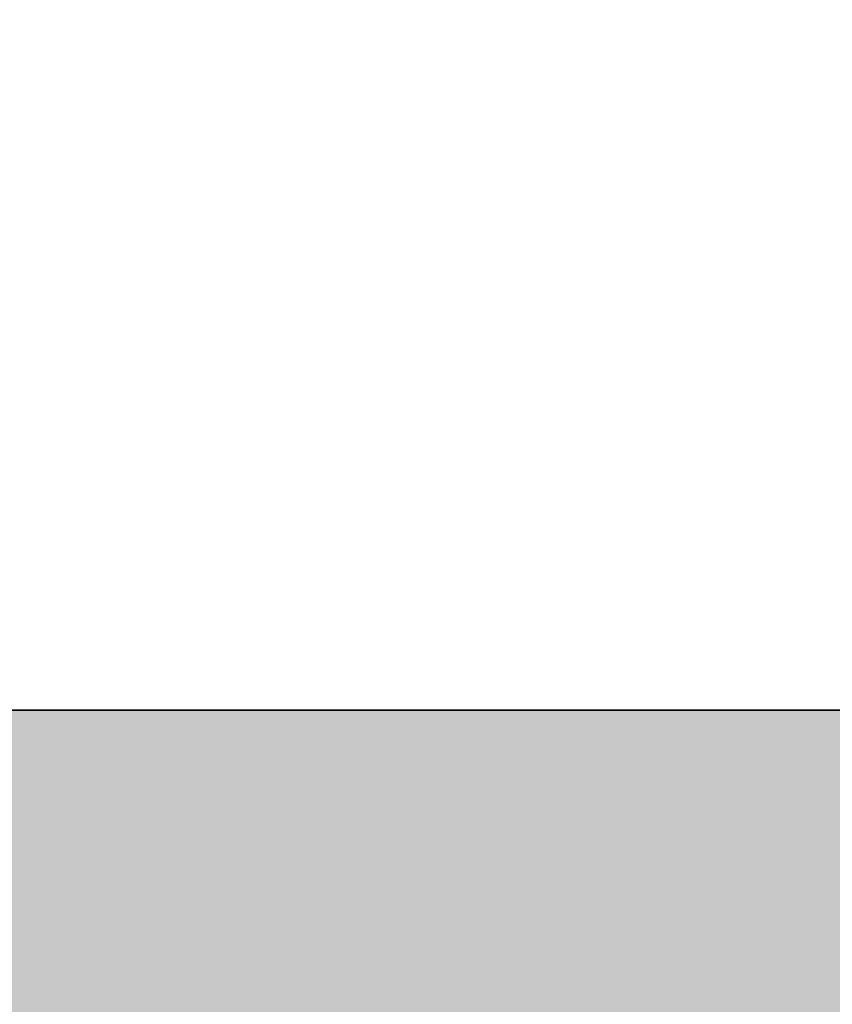
# Model space of a CAD drawing. Units: inches. Extents: x 2083 to 3317, y 1141 to 2115.
# Tile 24 of 256: x 2234.135 to 2235.918, y 1477.116 to 1479.275. Entities that reach past the tile are written whole.
import ezdxf

# ---------------------------------------------------------------- set-up
doc = ezdxf.new("R2010")
doc.units = ezdxf.units.IN
doc.layers.add('A-ANNO-DIMS', color=2, linetype='Continuous', lineweight=18)
doc.layers.add('A-WALL', color=7, linetype='Continuous', lineweight=35)
doc.layers.add('A-WALL-PATT', color=251, linetype='Continuous', lineweight=13, true_color=0x636466)
doc.styles.get("Standard").update_dxf_attribs({"font": 'arial.ttf'})
doc.dimstyles.new('ISO-25', dxfattribs={"dimtxt": 12, "dimasz": 12, "dimexe": 1.25, "dimexo": 0.625, "dimtad": 1, "dimlunit": 3, "dimtxsty": 'Standard', "dimcen": 2.5, "dimadec": 0, "dimazin": 0, "dimtfac": 1, "dimtmove": 0, "dimatfit": 3, "dimfxl": 1, "dimarcsym": 0})

# ---------------------------------------------------------------- blocks, each defined once
blk = doc.blocks.new('*D30')
at = {"layer": 'A-ANNO-DIMS', "color": 0, "lineweight": -2, "transparency": 16777216}
for p, q in [((2240.0179, 1445.2738), (2240.0179, 1448.0455)), ((2254.3293, 1445.2738), (2254.3293, 1448.0455)), ((2228.0179, 1446.7955), (2216.0179, 1446.7955)), ((2240.0179, 1446.7955), (2254.3293, 1446.7955)), ((2266.3293, 1446.7955), (2413.7649, 1446.7955))]:
    blk.add_line(p, q, dxfattribs=at)
at = {"layer": 'A-ANNO-DIMS', "color": 0, "transparency": 16777216}
for points in [[(2228.0179, 1448.7955), (2228.0179, 1444.7955), (2240.0179, 1446.7955)], [(2266.3293, 1448.7955), (2266.3293, 1444.7955), (2254.3293, 1446.7955)]]:
    blk.add_solid(points, dxfattribs=at)
at = {"layer": 'Defpoints', "color": 0, "transparency": 16777216}
for p in [(2254.3293, 1446.7955), (2240.0179, 1444.6488), (2254.3293, 1444.6488)]:
    blk.add_point(p, dxfattribs=at)
at = {"layer": 'A-ANNO-DIMS', "color": 0, "transparency": 16777216, "insert": (2346.0471, 1453.6252), "char_height": 12, "attachment_point": 5}
blk.add_mtext('WC 1\'-2 1/2" TYP.', dxfattribs=at)
blk = doc.blocks.new('*D31')
at = {"layer": 'A-ANNO-DIMS', "color": 0, "lineweight": -2, "transparency": 16777216}
for p, q in [((2237.8711, 1456.6488), (2237.8711, 1541.9152)), ((2239.3929, 1444.6488), (2236.6211, 1444.6488)), ((2237.8711, 1431.5475), (2237.8711, 1444.6488)), ((2239.3929, 1431.5475), (2236.6211, 1431.5475)), ((2237.8711, 1419.5475), (2237.8711, 1407.5475))]:
    blk.add_line(p, q, dxfattribs=at)
at = {"layer": 'A-ANNO-DIMS', "color": 0, "transparency": 16777216}
for points in [[(2235.8711, 1456.6488), (2239.8711, 1456.6488), (2237.8711, 1444.6488)], [(2235.8711, 1419.5475), (2239.8711, 1419.5475), (2237.8711, 1431.5475)]]:
    blk.add_solid(points, dxfattribs=at)
at = {"layer": 'Defpoints', "color": 0, "transparency": 16777216}
for p in [(2237.8711, 1444.6488), (2240.0179, 1444.6488), (2240.0179, 1431.5475)]:
    blk.add_point(p, dxfattribs=at)
at = {"layer": 'A-ANNO-DIMS', "color": 0, "transparency": 16777216, "insert": (2231.2175, 1505.282), "char_height": 12, "attachment_point": 5, "rotation": 90}
blk.add_mtext('1\'-1" TYP.', dxfattribs=at)

msp = doc.modelspace()

# ---------------------------------------------------------------- hatches: boundary and pattern name
at = {"layer": 'A-WALL-PATT'}
h = msp.add_hatch(color=256, dxfattribs=at)
h.dxf.hatch_style = 1
h.paths.add_polyline_path([(3126.9598, 2020.7614), (2748.9598, 2020.7614), (2604.9598, 2020.7614), (2226.9598, 2020.7614), (2226.9598, 1702.7614), (2466.9598, 1702.7614), (2466.9598, 1582.7614), (2418.9598, 1582.7614), (2418.9598, 1477.7614), (2226.9598, 1477.7614), (2226.9598, 1263.2614), (2544.9598, 1263.2614), (2544.9598, 1411.7614), (2604.9598, 1411.7614), (2685.9598, 1411.7614), (2685.9598, 1420.7614), (2604.9598, 1420.7614), (2604.9598, 1573.7614), (2604.9598, 1702.7614), (2604.9598, 2011.7614), (2748.9598, 2011.7614), (2748.9598, 1702.7614), (2862.9598, 1702.7614), (2862.9598, 1621.7614), (2871.9598, 1621.7614), (2871.9598, 1702.7614), (2883.9598, 1702.7614), (2883.9598, 1706.9395, -0.026459), (2883.9598, 1711.7614), (2757.9598, 1711.7614), (2757.9598, 1807.7614), (2787.9598, 1807.7614), (2787.9598, 1812.2614), (2757.9598, 1812.2614), (2757.9598, 2011.7614), (2877.9598, 2011.7614), (2877.9598, 1812.2614), (2847.9598, 1812.2614), (2847.9598, 1807.7614), (2889.8357, 1807.7614), (2889.8357, 1812.2614), (2882.4598, 1812.2614), (2882.4598, 2011.7614), (3117.9598, 2011.7614), (3117.9598, 1812.2614), (2937.8357, 1812.2614), (2937.8357, 1807.7614), (2995.7098, 1807.7614), (2995.7098, 1796.1177), (3000.2098, 1796.1177), (3000.2098, 1807.7614), (3117.9598, 1807.7614), (3117.9598, 1711.7614), (3000.2098, 1711.7614), (3000.2098, 1760.1177), (2998.5727, 1760.1177, -0.020711), (2995.7098, 1760.1177), (2995.7098, 1711.7614), (2931.9598, 1711.7614), (2931.9598, 1702.7614), (3126.9598, 1702.7614)])
h.paths.add_polyline_path([(2471.4598, 2011.7614), (2471.4598, 1810.0114), (2462.7169, 1810.0114), (2462.7169, 1805.5114), (2505.9598, 1805.5114), (2505.9598, 1810.0114), (2475.9598, 1810.0114), (2475.9598, 2011.7614), (2595.9598, 2011.7614), (2595.9598, 1810.0114), (2565.9598, 1810.0114), (2565.9598, 1805.5114), (2595.9598, 1805.5114), (2595.9598, 1711.7614), (2235.9598, 1711.7614), (2235.9598, 1805.5114), (2353.7098, 1805.5114), (2353.7098, 1796.0542), (2358.2098, 1796.0542), (2358.2098, 1805.5114), (2414.7169, 1805.5114), (2414.7169, 1810.0114), (2235.9598, 1810.0114), (2235.9598, 2011.7614)], flags=16)
h.paths.add_polyline_path([(2270.2047, 1994.61), (2270.2047, 1970.61), (2246.2047, 1970.61), (2246.2047, 1994.61)], flags=0)
edge = h.paths.add_edge_path(flags=0)
edge.add_ellipse((2332.0274, 1899.7982), major_axis=(-3.043, 3.043), ratio=0.168252, start_angle=-161.3322, end_angle=-156.3071, ccw=False)
edge.add_ellipse((2333.082, 1898.7435), major_axis=(-1.0546, 1.0546), ratio=0.453532, start_angle=-123.371, end_angle=-94.1591)
edge = h.paths.add_edge_path(flags=0)
edge.add_ellipse((2332.0274, 1968.8763), major_axis=(3.043, 3.043), ratio=0.168252, start_angle=18.6678, end_angle=23.6929)
edge.add_spline(control_points=[(2332.9256, 1970.6911), (2332.2268, 1970.3361), (2330.8937, 1969.6589), (2328.4131, 1970.9321), (2327.2039, 1967.7487), (2324.7096, 1969.9556), (2322.5328, 1967.0124), (2320.0128, 1971.2958), (2317.6803, 1968.1578), (2316.0405, 1967.102), (2315.4269, 1966.8096)], knot_values=[0, 0, 0, 0, 2.267059, 4.324559, 6.685584, 8.878641, 11.121502, 14.300359, 17.755284, 19.732645, 19.732645, 19.732645, 19.732645], degree=3, periodic=0)
edge.add_ellipse((2332.0274, 1968.8763), major_axis=(3.043, 3.043), ratio=0.168252, start_angle=18.6678, end_angle=23.6929, ccw=False)
edge.add_ellipse((2333.082, 1969.9309), major_axis=(1.0546, 1.0546), ratio=0.453532, start_angle=56.629, end_angle=85.8409, ccw=False)
edge = h.paths.add_edge_path(flags=0)
edge.add_spline(control_points=[(2296.4283, 1967.9879), (2293.6278, 1965.3363), (2287.7036, 1959.7271), (2299.7439, 1949.9957), (2294.5326, 1935.6685), (2290.5732, 1920.6035), (2293.3941, 1909.9737), (2296.1854, 1904.9665)], knot_values=[0.099185, 0.099185, 0.099185, 0.099185, 0.345301, 0.619822, 0.982653, 1.386093, 1.810555, 1.810555, 1.810555, 1.810555], degree=3, periodic=0)
edge.add_spline(control_points=[(2296.1854, 1904.9665), (2297.3836, 1902.6193), (2298.001, 1901.9493), (2298.553, 1901.4682)], knot_values=[0.006246, 0.006246, 0.006246, 0.006246, 0.055476, 0.055476, 0.055476, 0.055476], degree=3, periodic=0)
edge.add_spline(control_points=[(2298.553, 1901.4682), (2297.2586, 1900.9232), (2295.2253, 1900.2321), (2293.0602, 1900.6142), (2292.1014, 1900.7884), (2292.0896, 1900.7906)], knot_values=[0.312835, 0.312835, 0.312835, 0.312835, 0.40178, 0.474987, 0.475903, 0.475903, 0.475903, 0.475903], degree=3, periodic=0)
edge.add_arc((2292.7936, 1904.6641), 3.937, 215.4209, 259.6982, ccw=False)
edge.add_spline(control_points=[(2289.5853, 1902.3823), (2289.4767, 1902.5351), (2289.3685, 1902.688), (2289.2609, 1902.8412)], knot_values=[0.102872, 0.102872, 0.102872, 0.102872, 0.116896, 0.116896, 0.116896, 0.116896], degree=3, periodic=0)
edge.add_spline(control_points=[(2289.2609, 1902.8412), (2288.6866, 1902.5502), (2287.64, 1902.0199), (2285.8813, 1901.874), (2283.853, 1901.5044), (2281.72, 1899.7105), (2278.467, 1899.4929), (2276.1571, 1901.8832), (2272.259, 1899.8041), (2267.7776, 1901.8432), (2262.2439, 1900.184), (2257.4149, 1901.7821), (2254.3184, 1900.7261), (2253.1783, 1900.3373)], knot_values=[0, 0, 0, 0, 1.907977, 3.477176, 5.261074, 7.972851, 11.680248, 13.717921, 16.939592, 22.789562, 27.502503, 33.595215, 37.145618, 37.145618, 37.145618, 37.145618], degree=3, periodic=0)
edge.add_line((2253.1783, 1900.3373), (2250.2442, 1902.8412))
edge.add_line((2250.2442, 1902.8412), (2250.2442, 1965.8333))
edge.add_line((2250.2442, 1965.8333), (2253.1783, 1968.3371))
edge.add_spline(control_points=[(2253.1783, 1968.3371), (2254.3184, 1967.9483), (2257.4149, 1966.8924), (2262.2439, 1968.4904), (2267.7776, 1966.8313), (2271.5267, 1968.5372), (2273.8759, 1967.8283), (2274.2067, 1967.7276)], knot_values=[0, 0, 0, 0, 0.09018, 0.244935, 0.364644, 0.513233, 0.537855, 0.537855, 0.537855, 0.537855], degree=3, periodic=0)
edge.add_arc((2274.3529, 1963.7933), 3.937, 72.0511, 92.1279, ccw=False)
edge.add_arc((2281.2969, 1985.23), 18.5963, 252.05113, 288.56572)
edge.add_arc((2292.3167, 1956.0289), 12.6461, 71.02679, 113.77822, ccw=False)
edge = h.paths.add_edge_path(flags=0)
edge.add_spline(control_points=[(2274.8994, 1951.8562), (2275.0662, 1951.6166), (2275.2327, 1951.3766), (2275.398, 1951.1359)], knot_values=[1.409916, 1.409916, 1.409916, 1.409916, 1.43159, 1.43159, 1.43159, 1.43159], degree=3, periodic=0)
edge.add_spline(control_points=[(2275.398, 1951.1359), (2275.7921, 1950.5619), (2276.1792, 1949.9838), (2276.5455, 1949.3971)], knot_values=[1.358238, 1.358238, 1.358238, 1.358238, 1.409916, 1.409916, 1.409916, 1.409916], degree=3, periodic=0)
edge.add_line((2276.5455, 1949.3971), (2277.4373, 1947.8622))
edge.add_spline(control_points=[(2277.4373, 1947.8622), (2276.3038, 1945.6731), (2274.6397, 1942.4269), (2274.6316, 1938.0939), (2272.7991, 1930.8515), (2274.3564, 1943.897), (2275.9477, 1947.9234), (2276.5455, 1949.3971)], knot_values=[0.005632, 0.005632, 0.005632, 0.005632, 0.186014, 0.266002, 0.357087, 0.59639, 0.739732, 0.739732, 0.739732, 0.739732], degree=3, periodic=0)
edge.add_spline(control_points=[(2276.5455, 1949.3971), (2276.1792, 1949.9838), (2275.7921, 1950.5619), (2275.398, 1951.1359)], knot_values=[1.358238, 1.358238, 1.358238, 1.358238, 1.409916, 1.409916, 1.409916, 1.409916], degree=3, periodic=0)
edge.add_spline(control_points=[(2275.398, 1951.1359), (2274.9425, 1950.0805), (2274.2078, 1948.0253), (2273.9346, 1944.8515), (2272.4685, 1937.6275), (2273.4662, 1945.6965), (2274.7006, 1951.0595), (2274.8994, 1951.8562)], knot_values=[0.104364, 0.104364, 0.104364, 0.104364, 0.189636, 0.269624, 0.36071, 0.600013, 0.644622, 0.644622, 0.644622, 0.644622], degree=3, periodic=0)
h.paths.add_polyline_path([(2269.1675, 1963.1276, -0.357527), (2268.1706, 1960.9764, -0.092561), (2268.1706, 1939.4363, -0.357527), (2269.1675, 1937.2851, -0.357527), (2267.0163, 1938.282, -0.164785), (2254.6856, 1938.282, -0.357527), (2252.5344, 1937.2851, -0.357527), (2253.5313, 1939.4363, -0.092561), (2253.5313, 1960.9764, -0.357527), (2252.5344, 1963.1276, -0.357527), (2254.6856, 1962.1307, -0.164785), (2267.0163, 1962.1307, -0.357527)], flags=0)
h.paths.add_polyline_path([(2248.8741, 1967.8018), (2248.8741, 1957.0277), (2249.4578, 1957.0277), (2249.4578, 1911.6468), (2248.8741, 1911.6468), (2248.8741, 1900.8727), (2246.5119, 1900.8727, 0.197327), (2244.1497, 1902.4569), (2244.1497, 1966.2176, 0.197327), (2246.5119, 1967.8018)], flags=0)
h.paths.add_polyline_path([(2269.1675, 1931.3893, -0.357527), (2268.1706, 1929.2381, -0.092561), (2268.1706, 1907.6981, -0.357527), (2269.1675, 1905.5469, -0.357527), (2267.0163, 1906.5438, -0.164785), (2254.6856, 1906.5438, -0.357527), (2252.5344, 1905.5469, -0.357527), (2253.5313, 1907.6981, -0.092561), (2253.5313, 1929.2381, -0.357527), (2252.5344, 1931.3893, -0.357527), (2254.6856, 1930.3925, -0.164785), (2267.0163, 1930.3925, -0.357527)], flags=0)
edge = h.paths.add_edge_path(flags=0)
edge.add_spline(control_points=[(2276.1969, 1906.7237), (2276.1681, 1909.0289), (2276.114, 1913.3719), (2270.5984, 1924.925), (2273.9052, 1919.0128), (2275.9217, 1916.2621), (2275.4746, 1912.4021), (2277.2579, 1910.3806), (2276.696, 1908.225), (2276.6462, 1906.813), (2276.6178, 1906.0084)], knot_values=[0, 0, 0, 0, 8.61026, 16.221274, 18.843057, 23.804898, 27.440828, 29.356102, 31.203478, 33.650687, 33.650687, 33.650687, 33.650687], degree=3, periodic=0)
edge.add_spline(control_points=[(2276.6178, 1906.0084), (2276.6233, 1905.6241), (2276.4977, 1904.6287), (2275.4418, 1903.8547), (2274.9373, 1903.0804), (2274.8591, 1902.8412)], knot_values=[0.156488, 0.156488, 0.156488, 0.156488, 0.184398, 0.231376, 0.250598, 0.250598, 0.250598, 0.250598], degree=3, periodic=0)
edge.add_line((2274.8591, 1902.8412), (2276.506, 1902.8412))
edge.add_spline(control_points=[(2276.506, 1902.8412), (2276.7883, 1903.0849), (2277.6651, 1904.1252), (2278.2495, 1904.3407), (2277.6539, 1908.5274), (2278.1557, 1906.2278), (2278.1005, 1905.2859), (2278.8467, 1904.069), (2277.8568, 1903.4149), (2277.8742, 1902.991), (2277.9036, 1902.8412)], knot_values=[0.059574, 0.059574, 0.059574, 0.059574, 0.080753, 0.103741, 0.16972, 0.176036, 0.207137, 0.240474, 0.262341, 0.27366, 0.27366, 0.27366, 0.27366], degree=3, periodic=0)
edge.add_line((2277.9036, 1902.8412), (2280.0298, 1902.8412))
edge.add_spline(control_points=[(2280.0298, 1902.8412), (2279.8882, 1903.0884), (2279.4993, 1903.9816), (2280.1523, 1905.9393), (2278.1036, 1909.6578), (2279.7624, 1907.1853), (2280.3279, 1904.8749), (2280.4851, 1903.4896), (2281.4633, 1903.2494), (2281.7583, 1902.9365), (2281.834, 1902.8412)], knot_values=[0.013856, 0.013856, 0.013856, 0.013856, 0.034874, 0.088867, 0.107879, 0.126738, 0.158714, 0.193757, 0.217487, 0.226722, 0.226722, 0.226722, 0.226722], degree=3, periodic=0)
edge.add_spline(control_points=[(2281.834, 1902.8412), (2281.7875, 1902.8267), (2281.647, 1902.783), (2281.3955, 1902.8595), (2281.0881, 1902.9852), (2280.7207, 1903.0609), (2280.3335, 1903.0257), (2280.1248, 1902.8989), (2280.0298, 1902.8412)], knot_values=[0, 0, 0, 0, 0.14413, 0.435517, 0.749276, 1.153046, 1.548371, 1.878348, 1.878348, 1.878348, 1.878348], degree=3, periodic=0)
edge.add_line((2280.0298, 1902.8412), (2277.9036, 1902.8412))
edge.add_spline(control_points=[(2277.9036, 1902.8412), (2277.8929, 1902.7959), (2277.8654, 1902.6796), (2277.6075, 1902.6875), (2277.2741, 1902.8007), (2276.8379, 1902.6198), (2276.5838, 1902.7893), (2276.506, 1902.8412)], knot_values=[0, 0, 0, 0, 0.127189, 0.326199, 0.628009, 1.24357, 1.515331, 1.515331, 1.515331, 1.515331], degree=3, periodic=0)
edge.add_line((2276.506, 1902.8412), (2274.8591, 1902.8412))
edge.add_spline(control_points=[(2274.8591, 1902.8412), (2274.8144, 1902.8986), (2274.7251, 1903.0134), (2274.4935, 1903.119), (2274.2443, 1902.9605), (2273.9371, 1903.1849), (2273.614, 1902.9831), (2273.4083, 1902.883), (2273.3223, 1902.8412)], knot_values=[0, 0, 0, 0, 0.21843, 0.436957, 0.687977, 0.990379, 1.398396, 1.69185, 1.69185, 1.69185, 1.69185], degree=3, periodic=0)
edge.add_spline(control_points=[(2273.3223, 1902.8412), (2273.6167, 1903.4457), (2274.274, 1904.5383), (2276.0272, 1904.5737), (2276.207, 1906.5836), (2276.1969, 1906.7237)], knot_values=[0.012227, 0.012227, 0.012227, 0.012227, 0.059472, 0.106218, 0.134458, 0.134458, 0.134458, 0.134458], degree=3, periodic=0)
h.paths.add_polyline_path([(2270.7761, 1897.7898), (2270.7761, 1873.7898), (2246.7761, 1873.7898), (2246.7761, 1897.7898)], flags=0)
h.paths.add_polyline_path([(2353.7098, 1760.0051), (2353.7098, 1760.0542), (2358.2098, 1760.0542, -0.033729)], flags=0)
h.paths.add_polyline_path([(2321.8191, 1737.5292), (2341.9953, 1737.5292, -0.414214), (2343.2033, 1736.3212), (2343.2033, 1721.0206, -0.414214), (2341.9953, 1719.8127), (2321.8191, 1719.8127, -0.414214), (2320.6112, 1721.0206), (2320.6112, 1736.3212, -0.414214)], flags=0)
h.paths.add_polyline_path([(2324.235, 1736.3212), (2339.5794, 1736.3212, -0.414214), (2341.9953, 1733.9053), (2341.9953, 1725.4497, -0.414214), (2339.5794, 1723.0338), (2333.6806, 1723.0338), (2333.8453, 1722.0455, -0.870646), (2335.4254, 1721.8259, -0.767327), (2333.9227, 1721.4232), (2331.291, 1721.4232, -0.767327), (2329.7883, 1721.8259, -0.870646), (2331.3684, 1722.0455), (2331.5331, 1723.0338), (2324.235, 1723.0338, -0.414214), (2321.8191, 1725.4497), (2321.8191, 1733.9053, -0.414214)], flags=0)
h.paths.add_polyline_path([(2570.4838, 1928.6154), (2589.6838, 1928.6154), (2590.1688, 1928.6154), (2590.1688, 1904.9934), (2570.4838, 1904.9934)], flags=0)
h.paths.add_polyline_path([(2574.4473, 1927.2638, -1), (2572.8288, 1927.2638, -1)], flags=0)
h.paths.add_polyline_path([(2573.0899, 1926.9409), (2573.925, 1927.776), (2574.1477, 1927.5533), (2573.3126, 1926.7182)], flags=0)
h.paths.add_polyline_path([(2578.7791, 1919.7296, -1), (2571.5917, 1919.7296, -1)], flags=0)
h.paths.add_polyline_path([(2578.3854, 1919.7296, -1), (2571.9854, 1919.7296, -1)], flags=0)
h.paths.add_polyline_path([(2331.5958, 1729.4762, -1), (2333.618, 1729.4762, -1)], flags=0)
h.paths.add_polyline_path([(2578.0342, 1927.2638, -1), (2576.4157, 1927.2638, -1)], flags=0)
h.paths.add_polyline_path([(2576.6889, 1927.5311), (2576.9116, 1927.7538), (2577.7467, 1926.9186), (2577.524, 1926.6959)], flags=0)
h.paths.add_polyline_path([(2578.1391, 1909.8595, -1), (2572.2317, 1909.8595, -1)], flags=0)
h.paths.add_polyline_path([(2577.7454, 1909.8595, -1), (2572.6254, 1909.8595, -1)], flags=0)
h.paths.add_polyline_path([(2583.7977, 1927.2638, -1), (2582.1792, 1927.2638, -1)], flags=0)
h.paths.add_polyline_path([(2582.7186, 1927.7538), (2583.5538, 1926.9186), (2583.3311, 1926.6959), (2582.4959, 1927.5311)], flags=0)
h.paths.add_polyline_path([(2582.4959, 1927.5311), (2582.7186, 1927.7538), (2583.5538, 1926.9186), (2583.3311, 1926.6959)], flags=0)
h.paths.add_polyline_path([(2587.7391, 1920.5296, -1), (2581.8317, 1920.5296, -1)], flags=0)
h.paths.add_polyline_path([(2587.3454, 1920.5296, -1), (2582.2254, 1920.5296, -1)], flags=0)
h.paths.add_polyline_path([(2587.3846, 1927.2638, -1), (2585.7661, 1927.2638, -1)], flags=0)
h.paths.add_polyline_path([(2586.082, 1926.9802), (2586.9172, 1927.8154), (2587.1399, 1927.5927), (2586.3047, 1926.7575)], flags=0)
h.paths.add_polyline_path([(2588.3791, 1910.6595, -1), (2581.1917, 1910.6595, -1)], flags=0)
h.paths.add_polyline_path([(2587.9854, 1910.6595, -1), (2581.5854, 1910.6595, -1)], flags=0)
h.paths.add_polyline_path([(2417.1677, 1729.4779), (2437.3439, 1729.4779, -0.414214), (2438.5519, 1728.2699), (2438.5519, 1712.9693, -0.414214), (2437.3439, 1711.7614), (2417.1677, 1711.7614, -0.414214), (2415.9598, 1712.9693), (2415.9598, 1728.2699, -0.414214)], flags=0)
h.paths.add_polyline_path([(2419.5836, 1728.2699), (2434.928, 1728.2699, -0.414214), (2437.3439, 1725.8541), (2437.3439, 1717.3984, -0.414214), (2434.928, 1714.9825), (2429.0292, 1714.9825), (2429.1939, 1713.9942, -0.870646), (2430.774, 1713.7746, -0.767327), (2429.2713, 1713.372), (2426.6396, 1713.372, -0.767327), (2425.1369, 1713.7746, -0.870646), (2426.717, 1713.9942), (2426.8817, 1714.9825), (2419.5836, 1714.9825, -0.414214), (2417.1677, 1717.3984), (2417.1677, 1725.8541, -0.414214)], flags=0)
h.paths.add_polyline_path([(2419.5836, 1728.2699), (2434.928, 1728.2699, -0.414214), (2437.3439, 1725.8541), (2437.3439, 1717.3984, -0.414214), (2434.928, 1714.9825), (2429.0292, 1714.9825), (2428.3581, 1719.009), (2427.5528, 1719.009), (2426.8817, 1714.9825), (2419.5836, 1714.9825, -0.414214), (2417.1677, 1717.3984), (2417.1677, 1725.8541, -0.414214)], flags=0)
h.paths.add_polyline_path([(2426.9444, 1721.4249, -1), (2428.9666, 1721.4249, -1)], flags=0)
h.paths.add_polyline_path([(2475.9598, 1702.7614), (2595.9598, 1702.7614), (2595.9598, 1582.7614), (2475.9598, 1582.7614)], flags=16)
h.paths.add_polyline_path([(2427.9598, 1573.7614), (2595.9598, 1573.7614), (2595.9598, 1468.7614), (2595.9598, 1420.7614), (2384.4598, 1420.7614), (2384.4598, 1468.7614), (2427.9598, 1468.7614)], flags=16)
h.paths.add_polyline_path([(2379.9598, 1468.7614), (2379.9598, 1420.7614), (2235.9598, 1420.7614), (2235.9598, 1468.7614)], flags=16)
h.paths.add_polyline_path([(2317.816, 1466.6958), (2337.9922, 1466.6958, -0.414214), (2339.2002, 1465.4878), (2339.2002, 1450.1872, -0.414214), (2337.9922, 1448.9792), (2317.816, 1448.9792, -0.414214), (2316.6081, 1450.1872), (2316.6081, 1465.4878, -0.414214)], flags=0)
h.paths.add_polyline_path([(2320.2319, 1465.4878), (2335.5763, 1465.4878, -0.414214), (2337.9922, 1463.0719), (2337.9922, 1454.6163, -0.414214), (2335.5763, 1452.2004), (2329.6775, 1452.2004), (2329.8422, 1451.212, -0.870646), (2331.4223, 1450.9925, -0.767327), (2329.9196, 1450.5898), (2327.2879, 1450.5898, -0.767327), (2325.7852, 1450.9925, -0.870646), (2327.3653, 1451.212), (2327.53, 1452.2004), (2320.2319, 1452.2004, -0.414214), (2317.816, 1454.6163), (2317.816, 1463.0719, -0.414214)], flags=0)
h.paths.add_polyline_path([(2320.2319, 1465.4878), (2335.5763, 1465.4878, -0.414214), (2337.9922, 1463.0719), (2337.9922, 1454.6163, -0.414214), (2335.5763, 1452.2004), (2329.6775, 1452.2004), (2329.0064, 1456.2269), (2328.2011, 1456.2269), (2327.53, 1452.2004), (2320.2319, 1452.2004, -0.414214), (2317.816, 1454.6163), (2317.816, 1463.0719, -0.414214)], flags=0)
h.paths.add_polyline_path([(2327.5926, 1458.6428, -1), (2329.6148, 1458.6428, -1)], flags=0)
h.paths.add_polyline_path([(2244.4117, 1433.3405), (2241.9209, 1433.3405, -0.414214), (2240.0179, 1435.2435), (2240.0179, 1440.9528, -0.414211), (2241.9209, 1442.8559), (2244.4117, 1442.8559, -1.976472)], flags=0)
h.paths.add_polyline_path([(2245.3569, 1434.3975, -0.414214), (2245.3569, 1441.7988, -2.144098)], flags=0)
h.paths.add_polyline_path([(2535.9598, 1416.2614), (2535.9598, 1272.2614), (2235.9598, 1272.2614), (2235.9598, 1416.2614)], flags=16)
h.paths.add_polyline_path([(2260.1196, 1384.2928), (2260.1196, 1362.0386), (2237.8654, 1362.0386), (2237.8654, 1384.2928)], flags=0)
edge = h.paths.add_edge_path(flags=0)
edge.add_line((2318.2518, 1362.0933), (2318.1458, 1362.001))
edge.add_ellipse((2317.4451, 1360.431), major_axis=(2.8216, 2.8216), ratio=0.168252, start_angle=18.6678, end_angle=20.9481, ccw=False)
edge.add_ellipse((2318.423, 1361.409), major_axis=(0.9779, 0.9779), ratio=0.453532, start_angle=56.629, end_angle=70.2262, ccw=False)
edge = h.paths.add_edge_path(flags=0)
edge.add_line((2319.1074, 1295.5711), (2319.015, 1295.6771))
edge.add_ellipse((2317.4451, 1296.3778), major_axis=(-2.8216, 2.8216), ratio=0.168252, start_angle=-161.3322, end_angle=-159.0519, ccw=False)
edge.add_ellipse((2318.423, 1295.3999), major_axis=(-0.9779, 0.9779), ratio=0.453532, start_angle=-123.371, end_angle=-109.7738)
edge = h.paths.add_edge_path(flags=0)
edge.add_spline(control_points=[(2284.2103, 1301.1702), (2284.5807, 1300.4447), (2284.8912, 1299.892), (2285.1596, 1299.461)], knot_values=[0.039066, 0.039066, 0.039066, 0.039066, 0.055476, 0.055476, 0.055476, 0.055476], degree=3, periodic=0)
edge.add_line((2285.1596, 1299.461), (2284.2103, 1301.1702))
edge = h.paths.add_edge_path(flags=0)
edge.add_line((2280.4125, 1297.298), (2283.37, 1297.0361))
edge.add_line((2283.37, 1297.0361), (2286.4057, 1297.9263))
edge.add_spline(control_points=[(2286.4057, 1297.9263), (2285.3055, 1297.4631), (2284.3448, 1297.1292), (2283.37, 1297.0361)], knot_values=[0.394369, 0.394369, 0.394369, 0.394369, 0.475903, 0.475903, 0.475903, 0.475903], degree=3, periodic=0)
edge.add_spline(control_points=[(2283.37, 1297.0361), (2283.2814, 1297.0277), (2282.3163, 1296.9573), (2281.3125, 1297.1345), (2280.4234, 1297.296), (2280.4125, 1297.298)], knot_values=[0.312835, 0.312835, 0.312835, 0.312835, 0.320246, 0.393453, 0.394369, 0.394369, 0.394369, 0.394369], degree=3, periodic=0)
edge = h.paths.add_edge_path(flags=0)
edge.add_line((2284.4356, 1359.6073), (2280.4463, 1355.328))
edge.add_line((2280.4463, 1355.328), (2279.58, 1351.0178))
edge.add_line((2279.58, 1351.0178), (2282.413, 1346.5804))
edge.add_spline(control_points=[(2282.413, 1346.5804), (2283.1533, 1345.5892), (2284.2529, 1344.0289), (2284.801, 1342.3872), (2284.9352, 1341.8055)], knot_values=[1.240098, 1.240098, 1.240098, 1.240098, 1.332892, 1.382712, 1.382712, 1.382712, 1.382712], degree=3, periodic=0)
edge.add_spline(control_points=[(2284.9352, 1341.8055), (2285.3191, 1340.1406), (2285.233, 1338.4092), (2284.9099, 1336.6541)], knot_values=[1.097484, 1.097484, 1.097484, 1.097484, 1.240098, 1.240098, 1.240098, 1.240098], degree=3, periodic=0)
edge.add_spline(control_points=[(2284.9099, 1336.6541), (2284.5868, 1334.899), (2284.0267, 1333.1203), (2283.4626, 1331.3606)], knot_values=[0.95487, 0.95487, 0.95487, 0.95487, 1.097484, 1.097484, 1.097484, 1.097484], degree=3, periodic=0)
edge.add_line((2283.4626, 1331.3606), (2281.8904, 1326.1534))
edge.add_line((2281.8904, 1326.1534), (2280.7563, 1321.0561))
edge.add_line((2280.7563, 1321.0561), (2280.2992, 1316.002))
edge.add_line((2280.2992, 1316.002), (2280.7159, 1310.9501))
edge.add_line((2280.7159, 1310.9501), (2282.0281, 1305.9721))
edge.add_line((2282.0281, 1305.9721), (2284.2103, 1301.1702))
edge.add_spline(control_points=[(2284.2103, 1301.1702), (2283.3407, 1302.7302), (2282.6119, 1304.3365), (2282.0281, 1305.9721)], knot_values=[0.099185, 0.099185, 0.099185, 0.099185, 0.241799, 0.241799, 0.241799, 0.241799], degree=3, periodic=0)
edge.add_spline(control_points=[(2282.0281, 1305.9721), (2281.4443, 1307.6078), (2281.0055, 1309.2728), (2280.7159, 1310.9501)], knot_values=[0.241799, 0.241799, 0.241799, 0.241799, 0.384413, 0.384413, 0.384413, 0.384413], degree=3, periodic=0)
edge.add_spline(control_points=[(2280.7159, 1310.9501), (2280.4332, 1312.5876), (2280.2894, 1314.277), (2280.2989, 1315.962), (2280.2992, 1316.002)], knot_values=[0.384413, 0.384413, 0.384413, 0.384413, 0.523647, 0.527028, 0.527028, 0.527028, 0.527028], degree=3, periodic=0)
edge.add_spline(control_points=[(2280.2992, 1316.002), (2280.3123, 1317.687), (2280.4779, 1319.3679), (2280.7563, 1321.0561)], knot_values=[0.527028, 0.527028, 0.527028, 0.527028, 0.669642, 0.669642, 0.669642, 0.669642], degree=3, periodic=0)
edge.add_spline(control_points=[(2280.7563, 1321.0561), (2281.0346, 1322.7443), (2281.4259, 1324.4396), (2281.8904, 1326.1534)], knot_values=[0.669642, 0.669642, 0.669642, 0.669642, 0.812256, 0.812256, 0.812256, 0.812256], degree=3, periodic=0)
edge.add_spline(control_points=[(2281.8904, 1326.1534), (2282.2644, 1327.5333), (2282.7879, 1329.2618), (2283.3528, 1331.0178), (2283.4626, 1331.3606)], knot_values=[0.812256, 0.812256, 0.812256, 0.812256, 0.927087, 0.95487, 0.95487, 0.95487, 0.95487], degree=3, periodic=0)
edge.add_line((2283.4626, 1331.3606), (2284.9099, 1336.6541))
edge.add_line((2284.9099, 1336.6541), (2284.9352, 1341.8055))
edge.add_line((2284.9352, 1341.8055), (2282.413, 1346.5804))
edge.add_spline(control_points=[(2282.413, 1346.5804), (2281.2751, 1348.1038), (2280.0784, 1349.5703), (2279.58, 1351.0178)], knot_values=[1.382712, 1.382712, 1.382712, 1.382712, 1.525326, 1.525326, 1.525326, 1.525326], degree=3, periodic=0)
edge.add_spline(control_points=[(2279.58, 1351.0178), (2279.4433, 1351.4147), (2279.1363, 1352.8569), (2279.7352, 1354.2904), (2280.4463, 1355.328)], knot_values=[1.525326, 1.525326, 1.525326, 1.525326, 1.564439, 1.667941, 1.667941, 1.667941, 1.667941], degree=3, periodic=0)
edge.add_spline(control_points=[(2280.4463, 1355.328), (2281.4261, 1356.7578), (2282.9308, 1358.1826), (2284.4356, 1359.6073)], knot_values=[1.667941, 1.667941, 1.667941, 1.667941, 1.810555, 1.810555, 1.810555, 1.810555], degree=3, periodic=0)
edge.add_arc((2280.6231, 1348.5182), 11.7262, 71.02679, 113.77822)
edge.add_arc((2270.4049, 1375.5952), 17.2436, 252.05113, 288.56572, ccw=False)
edge.add_arc((2263.966, 1355.7178), 3.6506, 72.0511, 92.1279)
edge.add_arc((2263.966, 1355.7178), 3.6506, 92.1279, 177.9851)
edge.add_spline(control_points=[(2260.3176, 1355.8462), (2260.2604, 1354.2207), (2260.5513, 1350.1865), (2262.9993, 1346.7663), (2264.4727, 1344.649)], knot_values=[1.43159, 1.43159, 1.43159, 1.43159, 1.564144, 1.770695, 1.770695, 1.770695, 1.770695], degree=3, periodic=0)
edge.add_line((2264.4727, 1344.649), (2264.9356, 1343.9825))
edge.add_spline(control_points=[(2263.801, 1340.2481), (2263.8432, 1340.5141), (2264.0672, 1341.7565), (2264.5127, 1343.0025), (2264.935, 1343.9811)], knot_values=[0.53657, 0.53657, 0.53657, 0.53657, 0.559349, 0.644622, 0.644622, 0.644622, 0.644622], degree=3, periodic=0)
edge.add_spline(control_points=[(2264.935, 1343.9811), (2265.1178, 1343.715), (2265.2989, 1343.4479), (2265.4768, 1343.1794)], knot_values=[1.384077, 1.384077, 1.384077, 1.384077, 1.409916, 1.409916, 1.409916, 1.409916], degree=3, periodic=0)
edge.add_spline(control_points=[(2265.4768, 1343.1794), (2265.6546, 1342.9108), (2265.8293, 1342.6408), (2265.9991, 1342.3688)], knot_values=[1.358238, 1.358238, 1.358238, 1.358238, 1.384077, 1.384077, 1.384077, 1.384077], degree=3, periodic=0)
edge.add_line((2265.9991, 1342.3688), (2266.826, 1340.9455))
edge.add_spline(control_points=[(2266.826, 1340.9455), (2268.8944, 1337.0897), (2271.3982, 1325.843), (2270.5162, 1310.5686), (2275.9194, 1301.8606), (2277.7895, 1299.1994)], knot_values=[0.116896, 0.116896, 0.116896, 0.116896, 0.472987, 1.050969, 1.313793, 1.313793, 1.313793, 1.313793], degree=3, periodic=0)
edge.add_spline(control_points=[(2277.7895, 1299.1994), (2277.8394, 1299.1285), (2277.8894, 1299.0575), (2277.9396, 1298.9866)], knot_values=[0.109884, 0.109884, 0.109884, 0.109884, 0.116896, 0.116896, 0.116896, 0.116896], degree=3, periodic=0)
edge.add_line((2277.9396, 1298.9866), (2277.7888, 1299.1991))
edge.add_spline(control_points=[(2277.7888, 1299.1991), (2277.2566, 1298.9294), (2276.2864, 1298.4379), (2275.0394, 1298.3344), (2274.3833, 1298.2389), (2274.2153, 1298.2093)], knot_values=[33.12187, 33.12187, 33.12187, 33.12187, 35.029056, 36.598255, 37.144827, 37.144827, 37.144827, 37.144827], degree=3, periodic=0)
edge.add_line((2274.2153, 1298.2093), (2273.0731, 1297.893))
edge.add_spline(control_points=[(2273.0731, 1297.893), (2272.3229, 1297.5798), (2271.0392, 1296.5105), (2269.2484, 1296.2261), (2268.4231, 1296.3747)], knot_values=[26.532584, 26.532584, 26.532584, 26.532584, 29.198919, 31.839101, 31.839101, 31.839101, 31.839101], degree=3, periodic=0)
edge.add_line((2268.4231, 1296.3747), (2263.8785, 1297.4575))
edge.add_spline(control_points=[(2263.8785, 1297.4575), (2263.5561, 1297.3594), (2261.8603, 1296.8387), (2260.2388, 1297.2824), (2258.9335, 1297.5165)], knot_values=[15.919551, 15.919551, 15.919551, 15.919551, 16.939592, 21.226067, 21.226067, 21.226067, 21.226067], degree=3, periodic=0)
edge.add_line((2258.9335, 1297.5165), (2254.0552, 1297.329))
edge.add_spline(control_points=[(2254.0552, 1297.329), (2253.7555, 1297.2958), (2252.1137, 1297.1652), (2250.4619, 1297.5442), (2249.1297, 1297.6679)], knot_values=[5.306517, 5.306517, 5.306517, 5.306517, 6.276435, 10.613034, 10.613034, 10.613034, 10.613034], degree=3, periodic=0)
edge.add_line((2249.1297, 1297.6679), (2244.3316, 1296.8778))
edge.add_line((2244.3316, 1296.8778), (2241.611, 1299.1994))
edge.add_line((2241.611, 1299.1994), (2241.611, 1357.6094))
edge.add_line((2241.611, 1357.6094), (2244.3316, 1359.9311))
edge.add_line((2244.3316, 1359.9311), (2252.7288, 1359.5427))
edge.add_spline(control_points=[(2252.7288, 1359.5427), (2252.8709, 1359.5464), (2253.3057, 1359.5482), (2253.7398, 1359.5143), (2254.0317, 1359.4824)], knot_values=[0.233291, 0.233291, 0.233291, 0.233291, 0.244935, 0.268927, 0.268927, 0.268927, 0.268927], degree=3, periodic=0)
edge.add_line((2254.0317, 1359.4824), (2259.5872, 1359.4164))
edge.add_spline(control_points=[(2259.5872, 1359.4164), (2260.6771, 1359.6285), (2262.0732, 1359.897), (2263.5237, 1359.4593), (2263.8304, 1359.366)], knot_values=[0.422516, 0.422516, 0.422516, 0.422516, 0.513233, 0.537855, 0.537855, 0.537855, 0.537855], degree=3, periodic=0)
edge.add_arc((2263.966, 1355.7178), 3.6506, 72.0511, 92.1279, ccw=False)
edge.add_arc((2270.4049, 1375.5952), 17.2436, 252.05113, 288.56572)
edge.add_arc((2280.6231, 1348.5182), 11.7262, 71.02679, 113.77822, ccw=False)
h.paths.add_polyline_path([(2240.3405, 1359.4347), (2240.3405, 1349.4444), (2240.8818, 1349.4444), (2240.8818, 1307.3645), (2240.3405, 1307.3645), (2240.3405, 1297.3741), (2238.1502, 1297.3741, 0.197327), (2235.9598, 1298.8431), (2235.9598, 1357.9657, 0.197327), (2238.1502, 1359.4347)], flags=0)
h.paths.add_polyline_path([(2259.1578, 1355.1005, -0.357527), (2258.2334, 1353.1058, -0.092561), (2258.2334, 1333.1326, -0.357527), (2259.1578, 1331.1379, -0.357527), (2257.1631, 1332.0622, -0.164785), (2245.7293, 1332.0622, -0.357527), (2243.7346, 1331.1379, -0.357527), (2244.6589, 1333.1326, -0.092561), (2244.6589, 1353.1058, -0.357527), (2243.7346, 1355.1005, -0.357527), (2245.7293, 1354.1761, -0.164785), (2257.1631, 1354.1761, -0.357527)], flags=0)
edge = h.paths.add_edge_path(flags=0)
edge.add_line((2265.9991, 1342.3688), (2266.826, 1340.9455))
edge.add_line((2266.826, 1340.9455), (2265.3076, 1337.8141))
edge.add_line((2265.3076, 1337.8141), (2264.3582, 1334.6529))
edge.add_line((2264.3582, 1334.6529), (2264.262, 1333.7997))
edge.add_spline(control_points=[(2264.262, 1333.7997), (2264.2084, 1333.1871), (2264.1621, 1332.3655), (2264.0071, 1331.4139), (2263.969, 1331.2018)], knot_values=[0.464444, 0.464444, 0.464444, 0.464444, 0.516691, 0.531608, 0.531608, 0.531608, 0.531608], degree=3, periodic=0)
edge.add_spline(control_points=[(2263.969, 1331.2018), (2263.7745, 1330.1189), (2263.4244, 1328.7908), (2263.2574, 1328.5307), (2263.234, 1328.5146)], knot_values=[0.372682, 0.372682, 0.372682, 0.372682, 0.44885, 0.464444, 0.464444, 0.464444, 0.464444], degree=3, periodic=0)
edge.add_spline(control_points=[(2263.234, 1328.5146), (2263.0964, 1328.4202), (2263.1312, 1329.3015), (2263.275, 1330.6157)], knot_values=[0.280919, 0.280919, 0.280919, 0.280919, 0.372682, 0.372682, 0.372682, 0.372682], degree=3, periodic=0)
edge.add_spline(control_points=[(2263.275, 1330.6157), (2263.4187, 1331.93), (2263.6715, 1333.6773), (2263.9699, 1335.315)], knot_values=[0.189157, 0.189157, 0.189157, 0.189157, 0.280919, 0.280919, 0.280919, 0.280919], degree=3, periodic=0)
edge.add_spline(control_points=[(2263.9699, 1335.315), (2264.1005, 1336.0322), (2264.4188, 1337.6219), (2264.7548, 1338.8644), (2264.9474, 1339.4911)], knot_values=[0.097394, 0.097394, 0.097394, 0.097394, 0.137578, 0.189157, 0.189157, 0.189157, 0.189157], degree=3, periodic=0)
edge.add_spline(control_points=[(2264.9474, 1339.4911), (2265.29, 1340.6061), (2265.6442, 1341.494), (2265.9991, 1342.3688)], knot_values=[0.005632, 0.005632, 0.005632, 0.005632, 0.097394, 0.097394, 0.097394, 0.097394], degree=3, periodic=0)
h.paths.add_polyline_path([(2259.1578, 1325.671, -0.357527), (2258.2334, 1323.6763, -0.092561), (2258.2334, 1303.7031, -0.357527), (2259.1578, 1301.7084, -0.357527), (2257.1631, 1302.6327, -0.164785), (2245.7293, 1302.6327, -0.357527), (2243.7346, 1301.7084, -0.357527), (2244.6589, 1303.7031, -0.092561), (2244.6589, 1323.6763, -0.357527), (2243.7346, 1325.671, -0.357527), (2245.7293, 1324.7466, -0.164785), (2257.1631, 1324.7466, -0.357527)], flags=0)
edge = h.paths.add_edge_path(flags=0)
edge.add_spline(control_points=[(2261.7089, 1317.3114), (2261.6795, 1317.4176), (2261.7619, 1317.3885), (2262.4907, 1316.0899), (2262.9622, 1315.3009)], knot_values=[14.955861, 14.955861, 14.955861, 14.955861, 16.221274, 18.694826, 18.694826, 18.694826, 18.694826], degree=3, periodic=0)
edge.add_spline(control_points=[(2262.9622, 1315.3009), (2262.9904, 1315.2536), (2263.7021, 1314.0674), (2264.349, 1313.1272), (2264.7301, 1312.1642)], knot_values=[18.694826, 18.694826, 18.694826, 18.694826, 18.843057, 22.433791, 22.433791, 22.433791, 22.433791], degree=3, periodic=0)
edge.add_spline(control_points=[(2264.7301, 1312.1642), (2264.8756, 1311.7964), (2265.1769, 1310.7698), (2265.1431, 1309.5593), (2265.2477, 1308.8242)], knot_values=[22.433791, 22.433791, 22.433791, 22.433791, 23.804898, 26.172756, 26.172756, 26.172756, 26.172756], degree=3, periodic=0)
edge.add_line((2265.2477, 1308.8242), (2265.8508, 1307.1719))
edge.add_spline(control_points=[(2265.8508, 1307.1719), (2266.065, 1306.8217), (2266.3844, 1306.3322), (2266.4244, 1305.7805), (2266.4204, 1305.6112)], knot_values=[28.062562, 28.062562, 28.062562, 28.062562, 29.356102, 29.911721, 29.911721, 29.911721, 29.911721], degree=3, periodic=0)
edge.add_spline(control_points=[(2266.4204, 1305.6112), (2266.4161, 1305.4326), (2266.394, 1305.25), (2266.3648, 1305.0659)], knot_values=[29.911721, 29.911721, 29.911721, 29.911721, 30.497837, 30.497837, 30.497837, 30.497837], degree=3, periodic=0)
edge.add_line((2266.3648, 1305.0659), (2266.0662, 1302.1363))
edge.add_spline(control_points=[(2266.0662, 1302.1363), (2266.0712, 1301.78), (2265.9981, 1301.2), (2265.6633, 1300.759), (2265.5089, 1300.5859)], knot_values=[0.156488, 0.156488, 0.156488, 0.156488, 0.184398, 0.203543, 0.203543, 0.203543, 0.203543], degree=3, periodic=0)
edge.add_line((2265.5089, 1300.5859), (2264.4353, 1299.1994))
edge.add_line((2264.4353, 1299.1994), (2265.9624, 1299.1994))
edge.add_line((2265.9624, 1299.1994), (2267.336, 1301.1753))
edge.add_line((2267.336, 1301.1753), (2267.3117, 1301.9862))
edge.add_spline(control_points=[(2267.3117, 1301.9862), (2267.2611, 1302.8624), (2267.1602, 1303.7371), (2267.2715, 1303.3259)], knot_values=[0.126229, 0.126229, 0.126229, 0.126229, 0.166617, 0.166617, 0.166617, 0.166617], degree=3, periodic=0)
edge.add_spline(control_points=[(2267.2715, 1303.3259), (2267.28, 1303.2943), (2267.3098, 1303.1754), (2267.3735, 1302.8836), (2267.4061, 1302.6828), (2267.4179, 1302.601)], knot_values=[0.166617, 0.166617, 0.166617, 0.166617, 0.16972, 0.176036, 0.180765, 0.180765, 0.180765, 0.180765], degree=3, periodic=0)
edge.add_spline(control_points=[(2267.7439, 1300.9875), (2267.6876, 1301.1509), (2267.4805, 1301.6567), (2267.4838, 1302.1448), (2267.4179, 1302.601)], knot_values=[0.180765, 0.180765, 0.180765, 0.180765, 0.193767, 0.220139, 0.220139, 0.220139, 0.220139], degree=3, periodic=0)
edge.add_line((2267.4179, 1302.601), (2267.7439, 1300.9875))
edge.add_spline(control_points=[(2267.7439, 1300.9875), (2267.832, 1300.7319), (2267.932, 1300.3099), (2267.5548, 1299.9745), (2267.4294, 1299.8292)], knot_values=[0.220139, 0.220139, 0.220139, 0.220139, 0.240474, 0.25489, 0.25489, 0.25489, 0.25489], degree=3, periodic=0)
edge.add_line((2267.4294, 1299.8292), (2267.2584, 1299.1994))
edge.add_line((2267.2584, 1299.1994), (2269.23, 1299.1994))
edge.add_spline(control_points=[(2269.23, 1299.1994), (2269.0987, 1299.4287), (2268.8428, 1300.0163), (2269.0116, 1300.9159), (2268.9468, 1301.6607)], knot_values=[0.013856, 0.013856, 0.013856, 0.013856, 0.034874, 0.067073, 0.067073, 0.067073, 0.067073], degree=3, periodic=0)
edge.add_line((2268.9468, 1301.6607), (2268.4316, 1303.6031))
edge.add_spline(control_points=[(2268.4316, 1303.6031), (2268.1756, 1304.1924), (2267.5962, 1305.2513), (2268.0407, 1304.6232), (2268.2514, 1304.2824)], knot_values=[0.090155, 0.090155, 0.090155, 0.090155, 0.107879, 0.120289, 0.120289, 0.120289, 0.120289], degree=3, periodic=0)
edge.add_spline(control_points=[(2268.2514, 1304.2824), (2268.3609, 1304.1053), (2269.0578, 1302.918), (2269.3827, 1301.5904), (2269.5214, 1300.7759), (2269.5752, 1300.5558)], knot_values=[0.120289, 0.120289, 0.120289, 0.120289, 0.126738, 0.158714, 0.173506, 0.173506, 0.173506, 0.173506], degree=3, periodic=0)
edge.add_line((2269.5752, 1300.5558), (2270.6858, 1299.4213))
edge.add_spline(control_points=[(2270.6858, 1299.4213), (2270.7672, 1299.3573), (2270.8379, 1299.2814), (2270.9029, 1299.1994)], knot_values=[0.21816, 0.21816, 0.21816, 0.21816, 0.226722, 0.226722, 0.226722, 0.226722], degree=3, periodic=0)
edge.add_line((2270.9372, 1299.1929), (2270.9029, 1299.1994))
edge.add_spline(control_points=[(2270.9029, 1299.1994), (2270.8598, 1299.186), (2270.7295, 1299.1455), (2270.4963, 1299.2164), (2270.2717, 1299.3083), (2270.121, 1299.348), (2270.0633, 1299.3596)], knot_values=[0.939174, 0.939174, 0.939174, 0.939174, 1.083304, 1.374691, 1.68845, 1.878348, 1.878348, 1.878348, 1.878348], degree=3, periodic=0)
edge.add_line((2270.0633, 1299.3596), (2269.23, 1299.1994))
edge.add_line((2269.23, 1299.1994), (2267.2584, 1299.1994))
edge.add_spline(control_points=[(2267.2584, 1299.1994), (2267.2484, 1299.1574), (2267.223, 1299.0497), (2266.9838, 1299.0569), (2266.8092, 1299.1162), (2266.6769, 1299.1091), (2266.6365, 1299.1048)], knot_values=[0.757665, 0.757665, 0.757665, 0.757665, 0.884854, 1.083864, 1.385675, 1.515331, 1.515331, 1.515331, 1.515331], degree=3, periodic=0)
edge.add_spline(control_points=[(2266.6365, 1299.1048), (2266.4852, 1299.0888), (2266.2358, 1299.0171), (2266.0346, 1299.1513), (2265.9624, 1299.1994)], knot_values=[0, 0, 0, 0, 0.485905, 0.757665, 0.757665, 0.757665, 0.757665], degree=3, periodic=0)
edge.add_line((2265.9624, 1299.1994), (2264.4353, 1299.1994))
edge.add_line((2264.4353, 1299.1994), (2263.8584, 1299.3671))
edge.add_spline(control_points=[(2263.8584, 1299.3671), (2263.8189, 1299.3709), (2263.7795, 1299.3857), (2263.7401, 1299.4015)], knot_values=[0.845925, 0.845925, 0.845925, 0.845925, 0.978627, 0.978627, 0.978627, 0.978627], degree=3, periodic=0)
edge.add_line((2263.7218, 1299.3964), (2263.0103, 1299.1994))
edge.add_spline(control_points=[(2263.0103, 1299.1994), (2263.2458, 1299.6829), (2263.506, 1300.1281), (2263.8735, 1300.408)], knot_values=[0.012227, 0.012227, 0.012227, 0.012227, 0.052971, 0.052971, 0.052971, 0.052971], degree=3, periodic=0)
edge.add_spline(control_points=[(2263.8735, 1300.408), (2263.9321, 1300.4527), (2264.0842, 1300.553), (2264.2552, 1300.6242), (2264.3597, 1300.6647)], knot_values=[0.052971, 0.052971, 0.052971, 0.052971, 0.059472, 0.069086, 0.069086, 0.069086, 0.069086], degree=3, periodic=0)
edge.add_line((2264.3597, 1300.6647), (2265.1419, 1301.0778))
edge.add_line((2265.1419, 1301.0778), (2265.6758, 1302.7996))
edge.add_line((2265.6758, 1302.7996), (2265.5407, 1305.7041))
edge.add_line((2265.5407, 1305.7041), (2264.8031, 1309.3277))
edge.add_line((2264.8031, 1309.3277), (2263.0405, 1314.0918))
edge.add_spline(control_points=[(2263.0405, 1314.0918), (2262.3836, 1315.6714), (2261.796, 1316.9977), (2261.7089, 1317.3114)], knot_values=[11.216896, 11.216896, 11.216896, 11.216896, 14.955861, 14.955861, 14.955861, 14.955861], degree=3, periodic=0)
h.paths.add_polyline_path([(2871.9598, 1416.2614), (2895.91, 1416.2614), (2895.91, 1420.7614), (2871.9598, 1420.7614), (2871.9598, 1501.7614), (2862.9598, 1501.7614), (2862.9598, 1420.7614), (2805.9598, 1420.7614), (2805.9598, 1411.7614), (2862.9598, 1411.7614), (2862.9598, 1263.2614), (3126.9598, 1263.2614), (3126.9598, 1411.7614), (3126.9598, 1486.7614), (2943.9598, 1486.7614), (2943.9598, 1477.7614), (2967.8603, 1477.7614), (2967.8603, 1420.7614), (2943.91, 1420.7614), (2943.91, 1416.2614), (3117.9598, 1416.2614), (3117.9598, 1420.7614), (2972.3603, 1420.7614), (2972.3603, 1477.7614), (3117.9598, 1477.7614), (3117.9598, 1420.7614), (3117.9598, 1272.2614), (2871.9598, 1272.2614)], flags=0)
h.paths.add_polyline_path([(2457.1256, 1485.9425), (2527.6027, 1485.9425), (2527.6027, 1537.6357), (2457.1256, 1537.6357)], flags=8)
h.paths.add_polyline_path([(2481.0051, 1609.9818), (2590.7658, 1609.9818), (2590.7658, 1682.0034), (2481.0051, 1682.0034)], flags=8)
h.paths.add_polyline_path([(2483.085, 1729.1268), (2553.562, 1729.1268), (2553.562, 1780.82), (2483.085, 1780.82)], flags=8)

# ---------------------------------------------------------------- linework, layer by layer
at = {"layer": 'A-WALL'}
msp.add_line((2226.9598, 1477.7614), (2418.9598, 1477.7614), dxfattribs=at)

# ---------------------------------------------------------------- dimensions: what is measured, and where the dimension line sits
at = {"layer": 'A-ANNO-DIMS'}
dim = msp.add_linear_dim(base=(2237.8711, 1444.6488), p1=(2240.0179, 1431.5475), p2=(2240.0179, 1444.6488), angle=90, text='<> TYP.', dimstyle='ISO-25', override={"dimdec": 1, "dimlfac": 1, "dimrnd": 0, "dimzin": 1, "dimdsep": 46, "dimlunit": 4, "dimfrac": 2}, dxfattribs=at)
dim.commit()
dim.dimension.update_dxf_attribs({"geometry": '*D31', "text_midpoint": (2231.2175, 1505.282)})
dim = msp.add_linear_dim(base=(2254.3293, 1446.7955), p1=(2240.0179, 1444.6488), p2=(2254.3293, 1444.6488), text='WC <> TYP.', dimstyle='ISO-25', override={"dimdec": 1, "dimlfac": 1, "dimrnd": 0, "dimzin": 1, "dimdsep": 46, "dimlunit": 4, "dimfrac": 2}, dxfattribs=at)
dim.commit()
dim.dimension.update_dxf_attribs({"geometry": '*D30', "text_midpoint": (2346.0471, 1453.6252)})

doc.saveas('drawing.dxf')
